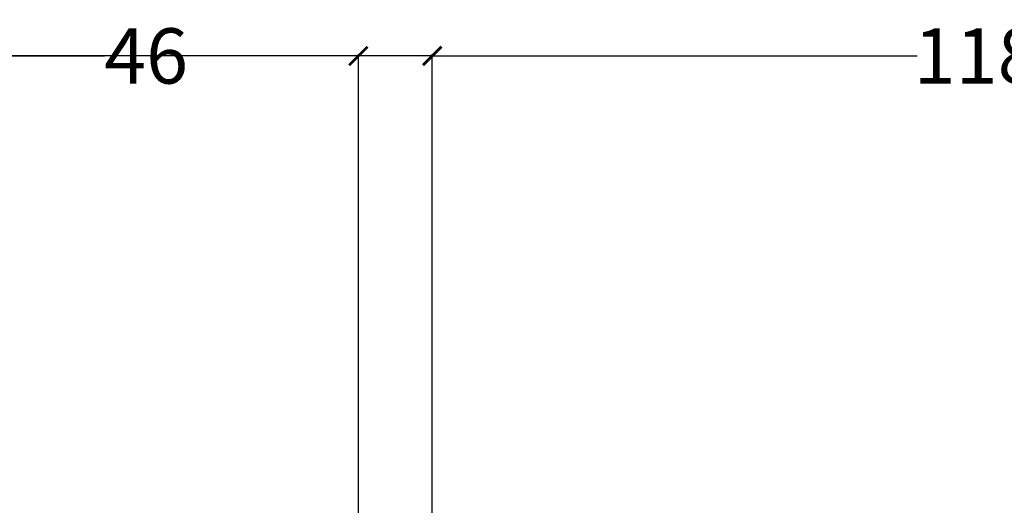
# Model space of a CAD drawing. Units: inches. Extents: x 1704 to 6393, y -157 to 1172.
# Tile 106 of 122: x 2561 to 2667, y 1056 to 1109. Entities that reach past the tile are written whole.
import ezdxf

# ---------------------------------------------------------------- set-up
doc = ezdxf.new("R2010")
doc.units = ezdxf.units.IN
doc.header["$MEASUREMENT"] = 0
doc.layers.add('A-ANNO-DIMS', color=7, linetype='Continuous', lineweight=13)
doc.styles.get("Standard").update_dxf_attribs({"font": 'arial.ttf'})
doc.dimstyles.get("Standard").update_dxf_attribs({"dimtxt": 6, "dimasz": 2, "dimexe": 0.18, "dimexo": 0.0625, "dimgap": 0.09, "dimtad": 0, "dimtih": 1, "dimtoh": 1, "dimdec": 1, "dimzin": 0, "dimdsep": 46, "dimlunit": 3, "dimtxsty": 'Standard', "dimblk": 'ARCHTICK', "dimcen": 0.09, "dimadec": 0, "dimazin": 0, "dimtfac": 1, "dimtdec": 1, "dimtofl": 0, "dimtmove": 0, "dimatfit": 3, "dimfxl": 1, "dimtolj": 1, "dimtzin": 0, "dimarcsym": 0})

# ---------------------------------------------------------------- blocks, each defined once
blk = doc.blocks.new('_ArchTick')
at = {"color": 0, "linetype": 'ByBlock', "const_width": 0.15}
blk.add_lwpolyline([(-0.5, -0.5), (0.5, 0.5)], dxfattribs=at)
blk = doc.blocks.new('*D92')
at = {"layer": 'A-ANNO-DIMS', "color": 0, "lineweight": -2, "transparency": 16777216}
for p, q in [((2073.35, 895.28), (2073.35, 1105.29)), ((2073.35, 1105.11), (2332.66, 1105.11)), ((2605.35, 1105.11), (2346.04, 1105.11)), ((2605.35, 895.28), (2605.35, 1105.29))]:
    blk.add_line(p, q, dxfattribs=at)
at = {"layer": 'Defpoints', "color": 0, "lineweight": -3, "transparency": 16777216}
for p in [(2605.35, 1105.11), (2073.35, 895.21), (2605.35, 895.21)]:
    blk.add_point(p, dxfattribs=at)
at = {"layer": 'A-ANNO-DIMS', "color": 0, "lineweight": -2, "transparency": 16777216, "xscale": 2, "yscale": 2, "zscale": 2, "rotation": 180}
blk.add_blockref('_ArchTick', (2073.35, 1105.11), dxfattribs=at)
at = {"layer": 'A-ANNO-DIMS', "color": 0, "lineweight": -2, "transparency": 16777216, "xscale": 2, "yscale": 2, "zscale": 2}
blk.add_blockref('_ArchTick', (2605.35, 1105.11), dxfattribs=at)
at = {"layer": 'A-ANNO-DIMS', "color": 0, "transparency": 16777216, "insert": (2339.35, 1105.11), "char_height": 6, "attachment_point": 5}
blk.add_mtext('\\A1;532', dxfattribs=at)
blk = doc.blocks.new('*D95')
at = {"layer": 'A-ANNO-DIMS', "color": 0, "lineweight": -2, "transparency": 16777216}
for p, q in [((2605.35, 895.28), (2605.35, 1105.29)), ((2605.35, 1105.11), (2657.91, 1105.11)), ((2723.35, 1105.11), (2670.79, 1105.11)), ((2723.35, 895.28), (2723.35, 1105.29))]:
    blk.add_line(p, q, dxfattribs=at)
at = {"layer": 'Defpoints', "color": 0, "lineweight": -3, "transparency": 16777216}
for p in [(2723.35, 1105.11), (2605.35, 895.21), (2723.35, 895.21)]:
    blk.add_point(p, dxfattribs=at)
at = {"layer": 'A-ANNO-DIMS', "color": 0, "lineweight": -2, "transparency": 16777216, "xscale": 2, "yscale": 2, "zscale": 2, "rotation": 180}
blk.add_blockref('_ArchTick', (2605.35, 1105.11), dxfattribs=at)
at = {"layer": 'A-ANNO-DIMS', "color": 0, "lineweight": -2, "transparency": 16777216, "xscale": 2, "yscale": 2, "zscale": 2}
blk.add_blockref('_ArchTick', (2723.35, 1105.11), dxfattribs=at)
at = {"layer": 'A-ANNO-DIMS', "color": 0, "transparency": 16777216, "insert": (2664.35, 1105.11), "char_height": 6, "attachment_point": 5}
blk.add_mtext('\\A1;118', dxfattribs=at)
blk = doc.blocks.new('*D103')
at = {"layer": 'A-ANNO-DIMS', "color": 0, "lineweight": -2, "transparency": 16777216}
for p, q in [((2551.35, 711.28), (2551.35, 1105.29)), ((2551.35, 1105.11), (2569.84, 1105.11)), ((2597.35, 1105.11), (2578.85, 1105.11)), ((2597.35, 711.28), (2597.35, 1105.29))]:
    blk.add_line(p, q, dxfattribs=at)
at = {"layer": 'Defpoints', "color": 0, "lineweight": -3, "transparency": 16777216}
for p in [(2597.35, 1105.11), (2551.35, 711.21), (2597.35, 711.21)]:
    blk.add_point(p, dxfattribs=at)
at = {"layer": 'A-ANNO-DIMS', "color": 0, "lineweight": -2, "transparency": 16777216, "xscale": 2, "yscale": 2, "zscale": 2, "rotation": 180}
blk.add_blockref('_ArchTick', (2551.35, 1105.11), dxfattribs=at)
at = {"layer": 'A-ANNO-DIMS', "color": 0, "lineweight": -2, "transparency": 16777216, "xscale": 2, "yscale": 2, "zscale": 2}
blk.add_blockref('_ArchTick', (2597.35, 1105.11), dxfattribs=at)
at = {"layer": 'A-ANNO-DIMS', "color": 0, "transparency": 16777216, "insert": (2574.35, 1105.11), "char_height": 6, "attachment_point": 5}
blk.add_mtext('\\A1;46', dxfattribs=at)

msp = doc.modelspace()

# ---------------------------------------------------------------- dimensions: what is measured, and where the dimension line sits
at = {"layer": 'A-ANNO-DIMS'}
for base, p1, p2, picture, middle in [((2605.349, 1105.107), (2073.349, 895.213), (2605.349, 895.213), '*D92', (2339.349, 1105.107)), ((2597.349, 1105.107), (2551.349, 711.213), (2597.349, 711.213), '*D103', (2574.349, 1105.107)), ((2723.349, 1105.107), (2605.349, 895.213), (2723.349, 895.213), '*D95', (2664.349, 1105.107))]:
    dim = msp.add_linear_dim(base=base, p1=p1, p2=p2, dimstyle='Standard', override={"dimdec": 0, "dimlfac": 1, "dimrnd": 0, "dimzin": 0, "dimdsep": 46, "dimlunit": 2}, dxfattribs=at)
    dim.commit()
    dim.dimension.update_dxf_attribs({"geometry": picture, "text_midpoint": middle})

doc.saveas('drawing.dxf')
